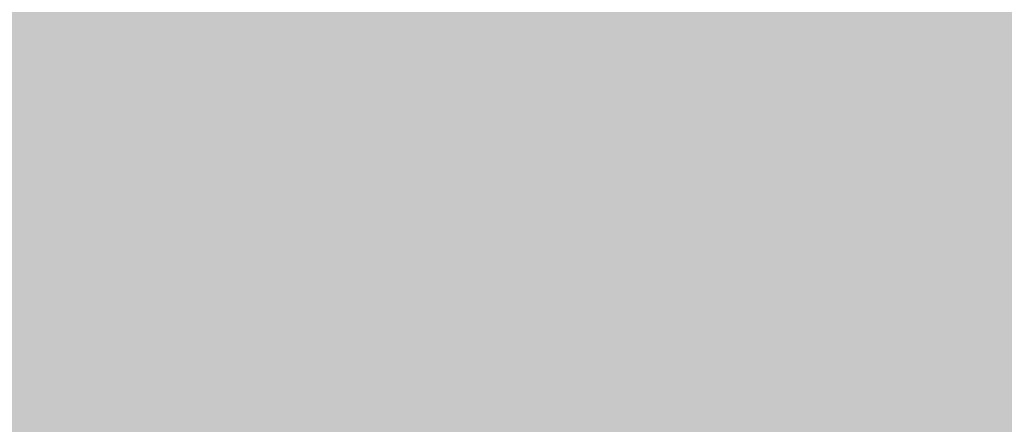
# Model space of a CAD drawing. Units: feet. Extents: x 3168 to 4724, y 827 to 1477.
# Tile 228 of 256: x 3379.08 to 3382.882, y 1096.781 to 1098.344. Entities that reach past the tile are written whole.
import ezdxf

# ---------------------------------------------------------------- set-up
doc = ezdxf.new("R2010")
doc.units = ezdxf.units.FT
doc.layers.add('A-ELEV-PATT', color=8, linetype='Continuous', lineweight=13)

msp = doc.modelspace()

# ---------------------------------------------------------------- hatches: boundary and pattern name
at = {"layer": 'A-ELEV-PATT'}
h = msp.add_hatch(color=256, dxfattribs=at)
h.dxf.hatch_style = 1
edge = h.paths.add_edge_path()
edge.add_ellipse((3552.9058, 979.2201), major_axis=(36.7449, 0), ratio=0.4848485, start_angle=0, end_angle=360)
edge = h.paths.add_edge_path()
edge.add_ellipse((3559.8916, 929.2523), major_axis=(36.7449, 0), ratio=0.4848485, start_angle=0, end_angle=360)
edge = h.paths.add_edge_path()
edge.add_line((3299.3168, 1198.6061), (3479.9167, 1198.6061))
edge.add_line((3479.9167, 1198.6061), (3479.9167, 1209.8686))
edge.add_spline(control_points=[(3479.9167, 1209.8686), (3464.3012, 1209.8686), (3448.6856, 1209.8686), (3410.9491, 1209.8686), (3388.8282, 1209.8686), (3355.6469, 1209.8686), (3344.5864, 1209.8686), (3327.9957, 1209.8686), (3322.4655, 1209.8686), (3314.1702, 1209.8686), (3311.4051, 1209.8686), (3307.2574, 1209.8686), (3305.8748, 1209.8686), (3303.801, 1209.8686), (3303.1097, 1209.8686), (3302.0728, 1209.8686), (3301.7272, 1209.8686), (3301.2087, 1209.8686), (3301.0359, 1209.8686), (3300.7767, 1209.8686), (3300.6903, 1209.8686), (3300.5606, 1209.8686), (3300.5174, 1209.8686), (3300.4526, 1209.8686), (3300.431, 1209.8686), (3300.3986, 1209.8686), (3300.3878, 1209.8686), (3300.3662, 1209.8686), (3300.3457, 1209.8686), (3300.3455, 1209.8686), (3300.3455, 1209.8686), (3300.3433, 1209.8686), (3300.3411, 1209.8686), (3300.3379, 1209.8686), (3300.3368, 1209.8686), (3300.3339, 1209.8686), (3300.3321, 1209.8686), (3300.3255, 1209.8686), (3300.3207, 1209.8686), (3300.3109, 1209.8686), (3300.306, 1209.8686), (3300.2905, 1209.8686), (3300.28, 1209.8686), (3300.2324, 1209.8688), (3300.1953, 1209.869), (3299.9511, 1209.8706), (3299.7448, 1209.8743), (3299.4368, 1209.8833), (3299.3344, 1209.8868), (3299.1811, 1209.8929), (3299.13, 1209.8951), (3298.6522, 1209.9168), (3298.2295, 1209.9457), (3297.6016, 1210.0024), (3297.3934, 1210.0235), (3297.0827, 1210.0583), (3296.9793, 1210.0705), (3296.293, 1210.1549), (3295.7181, 1210.2434), (3294.8687, 1210.3989), (3294.5877, 1210.4545), (3294.1693, 1210.5433), (3294.0304, 1210.5739), (3291.7071, 1211.1012), (3289.6536, 1211.8134), (3285.7763, 1213.564), (3283.9514, 1214.6035), (3280.5122, 1216.9801), (3278.8972, 1218.3176), (3276.3799, 1220.8295), (3275.416, 1221.9177), (3274.0393, 1223.7077), (3273.581, 1224.3495), (3273.1432, 1225.0163)], knot_values=[39.119033, 39.119033, 39.119033, 39.119033, 39.286353, 39.286353, 39.523379, 39.523379, 39.641892, 39.641892, 39.701148, 39.701148, 39.730777, 39.730777, 39.745591, 39.745591, 39.752998, 39.752998, 39.756701, 39.756701, 39.758553, 39.758553, 39.759479, 39.759479, 39.759942, 39.759942, 39.760173, 39.760173, 39.760289, 39.760289, 39.760405, 39.760405, 39.760463, 39.760463, 39.763389, 39.763389, 39.764851, 39.764851, 39.767304, 39.767304, 39.773825, 39.773825, 39.78057, 39.78057, 39.79477, 39.79477, 39.845194, 39.845194, 40.126715, 40.126715, 40.267476, 40.267476, 40.337856, 40.337856, 40.927023, 40.927023, 41.221606, 41.221606, 41.368898, 41.368898, 42.202622, 42.202622, 42.619485, 42.619485, 42.827916, 42.827916, 46.118323, 46.118323, 49.408731, 49.408731, 52.699139, 52.699139, 54.927489, 54.927489, 56.104228, 56.104228, 56.104228, 56.104228], weights=[1, 1, 1, 1, 1, 1, 1, 1, 1, 1, 1, 1, 1, 1, 1, 1, 1, 1, 1, 1, 1, 1, 1, 1, 1, 1, 1, 1, 1, 1, 1, 1, 1, 1, 1, 1, 1, 1, 1, 1, 1, 1, 1, 1, 1, 1, 1, 1, 1, 1, 1, 1, 1, 1, 1, 1, 1, 1, 1, 1, 1, 1, 1, 1, 1, 1, 1, 1, 1, 1, 1, 1, 1, 1], degree=3, periodic=0)
edge.add_line((3273.1432, 1225.0163), (3273.1432, 1099.0163))
edge.add_line((3273.1432, 1099.0163), (3299.3168, 1099.0163))
edge.add_line((3299.3168, 1099.0163), (3299.3168, 1198.6061))
edge = h.paths.add_edge_path()
edge.add_line((3304.7584, 1324.1581), (3479.9167, 1324.1581))
edge.add_line((3479.9167, 1324.1581), (3479.9167, 1335.7146))
edge.add_line((3479.9167, 1335.7146), (3269.1616, 1335.7146))
edge.add_spline(control_points=[(3269.1616, 1335.7146), (3264.0242, 1335.7146), (3258.3641, 1328.9582), (3259.2643, 1323.9003)], knot_values=[0, 0, 0, 0, 15.412191, 15.412191, 15.412191, 15.412191], degree=3, periodic=0)
edge.add_line((3259.2643, 1323.9003), (3265.5168, 1288.7691))
edge.add_line((3265.5168, 1288.7691), (3275.2651, 1261.5456))
edge.add_line((3275.2651, 1261.5456), (3304.7584, 1261.5456))
edge.add_line((3304.7584, 1261.5456), (3304.7584, 1324.1581))
h = msp.add_hatch(color=256, dxfattribs=at)
h.dxf.hatch_style = 1
h.paths.add_polyline_path([(3384.5252, 1099.0163), (3335.0292, 1099.0163), (3299.3168, 1099.0163), (3273.1432, 1099.0163), (3217.5654, 1099.0163), (3168.0693, 827.1163), (3335.0292, 827.1163)])

doc.saveas('drawing.dxf')
